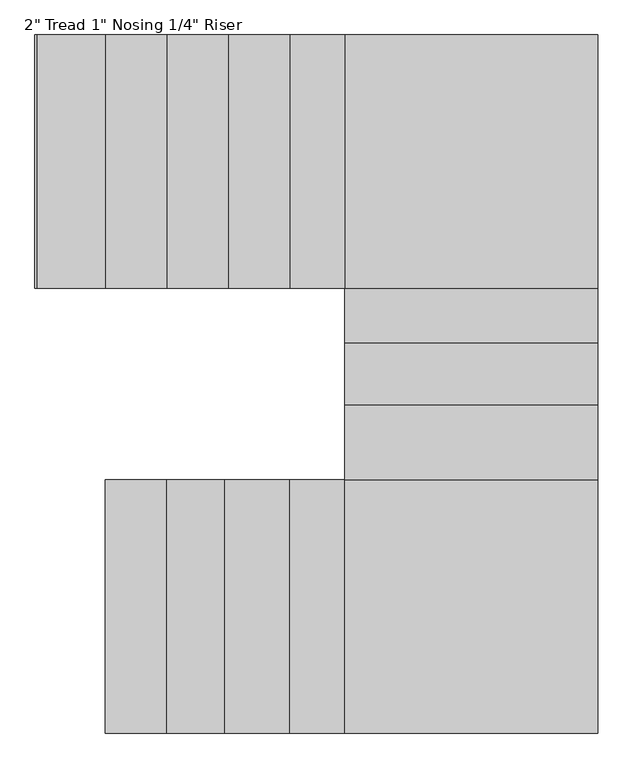
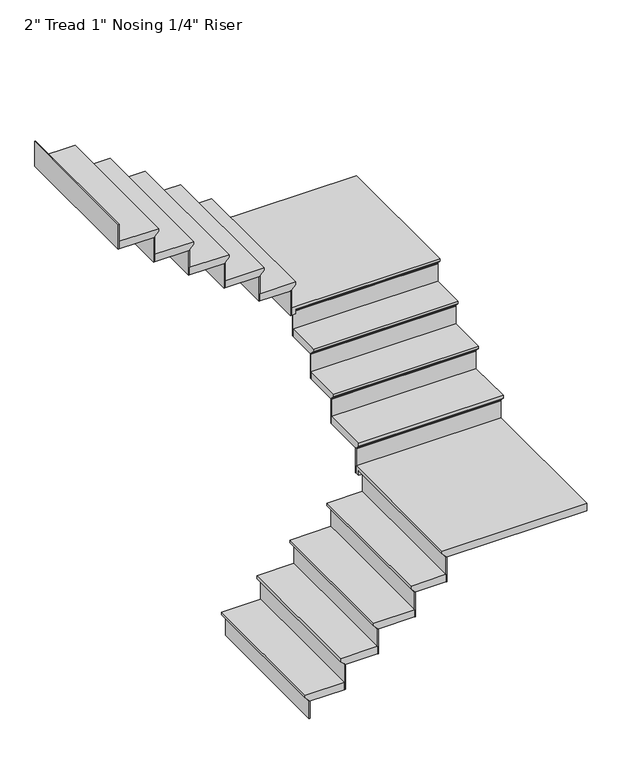
"""IFC4 building model written with IfcOpenShell, lengths in millimetres: stair flight geometry."""

from ifc_helpers import new_model, si_unit, origin, place, context, project, spatial, faceted_brep, source, transform, mapped, element, save


def stair_flight_84673ee4(model_context):
    return source(origin(), model_context, "Body", "Brep", [
        faceted_brep([(344.764115, -6141.1350571, 3350.6833333), (344.764115, -6141.1350571, 3369.7333333), (344.764115, -5201.3350571, 3369.7333333), (344.764115, -5201.3350571, 3350.6833333), (370.164115, -6141.1350571, 3325.2833333), (370.164115, -5201.3350571, 3325.2833333), (598.764115, -6141.1350571, 3369.7333333), (598.764115, -5201.3350571, 3369.7333333), (370.164115, -5201.3350571, 3318.9333333), (598.764115, -5201.3350571, 3318.9333333), (598.764115, -6141.1350571, 3318.9333333), (370.164115, -6141.1350571, 3318.9333333)], [[[0, 1, 2, 3]], [[4, 0, 3, 5]], [[2, 1, 6, 7]], [[8, 9, 10, 11]], [[2, 7, 9, 8, 5, 3]], [[8, 11, 4, 5]], [[6, 1, 0, 4, 11, 10]], [[7, 6, 10, 9]]]),
        faceted_brep([(370.164115, -6141.1350571, 3318.9333333), (370.164115, -6141.1350571, 3200.4), (376.514115, -6141.1350571, 3200.4), (376.514115, -6141.1350571, 3318.9333333), (370.164115, -5201.3350571, 3318.9333333), (376.514115, -5201.3350571, 3318.9333333), (376.514115, -5201.3350571, 3200.4), (370.164115, -5201.3350571, 3200.4)], [[[0, 1, 2, 3]], [[4, 5, 6, 7]], [[1, 0, 4, 7]], [[2, 1, 7, 6]], [[3, 2, 6, 5]], [[0, 3, 5, 4]]]),
        faceted_brep([(598.764115, -6141.1350571, 3488.2666667), (598.764115, -6141.1350571, 3318.9333333), (605.114115, -6141.1350571, 3318.9333333), (605.114115, -6141.1350571, 3488.2666667), (598.764115, -5201.3350571, 3488.2666667), (605.114115, -5201.3350571, 3488.2666667), (605.114115, -5201.3350571, 3318.9333333), (598.764115, -5201.3350571, 3318.9333333)], [[[0, 1, 2, 3]], [[4, 5, 6, 7]], [[1, 0, 4, 7]], [[2, 1, 7, 6]], [[3, 2, 6, 5]], [[0, 3, 5, 4]]]),
        faceted_brep([(573.364115, -5201.3350571, 3539.0666667), (573.364115, -6141.1350571, 3539.0666667), (814.664115, -6141.1350571, 3539.0666667), (814.664115, -5201.3350571, 3539.0666667), (598.764115, -5201.3350571, 3488.2666667), (814.664115, -5201.3350571, 3488.2666667), (814.664115, -6141.1350571, 3488.2666667), (598.764115, -6141.1350571, 3488.2666667), (598.764115, -5201.3350571, 3494.6166667), (573.364115, -5201.3350571, 3520.0166667), (598.764115, -6141.1350571, 3494.6166667), (573.364115, -6141.1350571, 3520.0166667)], [[[0, 1, 2, 3]], [[4, 5, 6, 7]], [[0, 3, 5, 4, 8, 9]], [[4, 7, 10, 8]], [[2, 1, 11, 10, 7, 6]], [[3, 2, 6, 5]], [[11, 1, 0, 9]], [[10, 11, 9, 8]]]),
        faceted_brep([(814.664115, -6141.1350571, 3657.6), (814.664115, -6141.1350571, 3488.2666667), (821.014115, -6141.1350571, 3488.2666667), (821.014115, -6141.1350571, 3657.6), (814.664115, -5201.3350571, 3657.6), (821.014115, -5201.3350571, 3657.6), (821.014115, -5201.3350571, 3488.2666667), (814.664115, -5201.3350571, 3488.2666667)], [[[0, 1, 2, 3]], [[4, 5, 6, 7]], [[1, 0, 4, 7]], [[2, 1, 7, 6]], [[3, 2, 6, 5]], [[0, 3, 5, 4]]]),
        faceted_brep([(789.264115, -5201.3350571, 3708.4), (789.264115, -6141.1350571, 3708.4), (1055.964115, -6141.1350571, 3708.4), (1055.964115, -5201.3350571, 3708.4), (814.664115, -5201.3350571, 3657.6), (1055.964115, -5201.3350571, 3657.6), (1055.964115, -6141.1350571, 3657.6), (814.664115, -6141.1350571, 3657.6), (814.664115, -5201.3350571, 3663.95), (789.264115, -5201.3350571, 3689.35), (814.664115, -6141.1350571, 3663.95), (789.264115, -6141.1350571, 3689.35)], [[[0, 1, 2, 3]], [[4, 5, 6, 7]], [[0, 3, 5, 4, 8, 9]], [[4, 7, 10, 8]], [[2, 1, 11, 10, 7, 6]], [[3, 2, 6, 5]], [[11, 1, 0, 9]], [[10, 11, 9, 8]]]),
        faceted_brep([(1055.964115, -6141.1350571, 3826.9333333), (1055.964115, -6141.1350571, 3657.6), (1062.314115, -6141.1350571, 3657.6), (1062.314115, -6141.1350571, 3826.9333333), (1055.964115, -5201.3350571, 3826.9333333), (1062.314115, -5201.3350571, 3826.9333333), (1062.314115, -5201.3350571, 3657.6), (1055.964115, -5201.3350571, 3657.6)], [[[0, 1, 2, 3]], [[4, 5, 6, 7]], [[1, 0, 4, 7]], [[2, 1, 7, 6]], [[3, 2, 6, 5]], [[0, 3, 5, 4]]]),
        faceted_brep([(1030.564115, -5201.3350571, 3877.7333333), (1030.564115, -6141.1350571, 3877.7333333), (1259.164115, -6141.1350571, 3877.7333333), (1259.164115, -5201.3350571, 3877.7333333), (1055.964115, -5201.3350571, 3826.9333333), (1259.164115, -5201.3350571, 3826.9333333), (1259.164115, -6141.1350571, 3826.9333333), (1055.964115, -6141.1350571, 3826.9333333), (1055.964115, -5201.3350571, 3833.2833333), (1030.564115, -5201.3350571, 3858.6833333), (1055.964115, -6141.1350571, 3833.2833333), (1030.564115, -6141.1350571, 3858.6833333)], [[[0, 1, 2, 3]], [[4, 5, 6, 7]], [[0, 3, 5, 4, 8, 9]], [[4, 7, 10, 8]], [[2, 1, 11, 10, 7, 6]], [[3, 2, 6, 5]], [[11, 1, 0, 9]], [[10, 11, 9, 8]]]),
        faceted_brep([(1259.164115, -6141.1350571, 3996.2666667), (1259.164115, -6141.1350571, 3826.9333333), (1265.514115, -6141.1350571, 3826.9333333), (1265.514115, -6141.1350571, 3996.2666667), (1259.164115, -5201.3350571, 3996.2666667), (1265.514115, -5201.3350571, 3996.2666667), (1265.514115, -5201.3350571, 3826.9333333), (1259.164115, -5201.3350571, 3826.9333333)], [[[0, 1, 2, 3]], [[4, 5, 6, 7]], [[1, 0, 4, 7]], [[2, 1, 7, 6]], [[3, 2, 6, 5]], [[0, 3, 5, 4]]]),
        faceted_brep([(2173.564115, -6141.1350571, 4047.0666667), (2173.564115, -5175.9350571, 4047.0666667), (1233.764115, -5175.9350571, 4047.0666667), (1233.764115, -6141.1350571, 4047.0666667), (1233.764115, -5201.3350571, 3996.2666667), (1233.764115, -5175.9350571, 3996.2666667), (2173.564115, -5175.9350571, 3996.2666667), (2173.564115, -6141.1350571, 3996.2666667), (1259.164115, -6141.1350571, 3996.2666667), (1259.164115, -5201.3350571, 3996.2666667), (1233.764115, -5201.3350571, 4028.0166667), (1233.764115, -6141.1350571, 4028.0166667), (1259.164115, -5201.3350571, 4002.6166667), (1259.164115, -6141.1350571, 4002.6166667)], [[[0, 1, 2, 3]], [[4, 5, 6, 7, 8, 9]], [[3, 2, 5, 4, 10, 11]], [[4, 9, 12, 10]], [[9, 8, 13, 12]], [[0, 3, 11, 13, 8, 7]], [[1, 0, 7, 6]], [[2, 1, 6, 5]], [[13, 11, 10, 12]]]),
        faceted_brep([(2173.564115, -5175.9350571, 4165.6), (2173.564115, -5175.9350571, 3996.2666667), (2173.564115, -5169.5850571, 3996.2666667), (2173.564115, -5169.5850571, 4165.6), (1233.764115, -5175.9350571, 4165.6), (1233.764115, -5169.5850571, 4165.6), (1233.764115, -5169.5850571, 3996.2666667), (1233.764115, -5175.9350571, 3996.2666667)], [[[0, 1, 2, 3]], [[4, 5, 6, 7]], [[1, 0, 4, 7]], [[2, 1, 7, 6]], [[3, 2, 6, 5]], [[0, 3, 5, 4]]]),
        faceted_brep([(1233.764115, -5201.3350571, 4216.4), (2173.564115, -5201.3350571, 4216.4), (2173.564115, -4896.5350571, 4216.4), (1233.764115, -4896.5350571, 4216.4), (1233.764115, -5175.9350571, 4165.6), (1233.764115, -4896.5350571, 4165.6), (2173.564115, -4896.5350571, 4165.6), (2173.564115, -5175.9350571, 4165.6), (1233.764115, -5175.9350571, 4171.95), (1233.764115, -5201.3350571, 4197.35), (2173.564115, -5175.9350571, 4171.95), (2173.564115, -5201.3350571, 4197.35)], [[[0, 1, 2, 3]], [[4, 5, 6, 7]], [[0, 3, 5, 4, 8, 9]], [[4, 7, 10, 8]], [[2, 1, 11, 10, 7, 6]], [[3, 2, 6, 5]], [[11, 1, 0, 9]], [[10, 11, 9, 8]]]),
        faceted_brep([(2173.564115, -4896.5350571, 4334.9333333), (2173.564115, -4896.5350571, 4165.6), (2173.564115, -4890.1850571, 4165.6), (2173.564115, -4890.1850571, 4334.9333333), (1233.764115, -4896.5350571, 4334.9333333), (1233.764115, -4890.1850571, 4334.9333333), (1233.764115, -4890.1850571, 4165.6), (1233.764115, -4896.5350571, 4165.6)], [[[0, 1, 2, 3]], [[4, 5, 6, 7]], [[1, 0, 4, 7]], [[2, 1, 7, 6]], [[3, 2, 6, 5]], [[0, 3, 5, 4]]]),
        faceted_brep([(1233.764115, -4921.9350571, 4385.7333333), (2173.564115, -4921.9350571, 4385.7333333), (2173.564115, -4667.9350571, 4385.7333333), (1233.764115, -4667.9350571, 4385.7333333), (1233.764115, -4896.5350571, 4334.9333333), (1233.764115, -4667.9350571, 4334.9333333), (2173.564115, -4667.9350571, 4334.9333333), (2173.564115, -4896.5350571, 4334.9333333), (1233.764115, -4896.5350571, 4341.2833333), (1233.764115, -4921.9350571, 4366.6833333), (2173.564115, -4896.5350571, 4341.2833333), (2173.564115, -4921.9350571, 4366.6833333)], [[[0, 1, 2, 3]], [[4, 5, 6, 7]], [[0, 3, 5, 4, 8, 9]], [[4, 7, 10, 8]], [[2, 1, 11, 10, 7, 6]], [[3, 2, 6, 5]], [[11, 1, 0, 9]], [[10, 11, 9, 8]]]),
        faceted_brep([(2173.564115, -4667.9350571, 4504.2666667), (2173.564115, -4667.9350571, 4334.9333333), (2173.564115, -4661.5850571, 4334.9333333), (2173.564115, -4661.5850571, 4504.2666667), (1233.764115, -4667.9350571, 4504.2666667), (1233.764115, -4661.5850571, 4504.2666667), (1233.764115, -4661.5850571, 4334.9333333), (1233.764115, -4667.9350571, 4334.9333333)], [[[0, 1, 2, 3]], [[4, 5, 6, 7]], [[1, 0, 4, 7]], [[2, 1, 7, 6]], [[3, 2, 6, 5]], [[0, 3, 5, 4]]]),
        faceted_brep([(1233.764115, -4693.3350571, 4555.0666667), (2173.564115, -4693.3350571, 4555.0666667), (2173.564115, -4464.7350571, 4555.0666667), (1233.764115, -4464.7350571, 4555.0666667), (1233.764115, -4667.9350571, 4504.2666667), (1233.764115, -4464.7350571, 4504.2666667), (2173.564115, -4464.7350571, 4504.2666667), (2173.564115, -4667.9350571, 4504.2666667), (1233.764115, -4667.9350571, 4510.6166667), (1233.764115, -4693.3350571, 4536.0166667), (2173.564115, -4667.9350571, 4510.6166667), (2173.564115, -4693.3350571, 4536.0166667)], [[[0, 1, 2, 3]], [[4, 5, 6, 7]], [[0, 3, 5, 4, 8, 9]], [[4, 7, 10, 8]], [[2, 1, 11, 10, 7, 6]], [[3, 2, 6, 5]], [[11, 1, 0, 9]], [[10, 11, 9, 8]]]),
        faceted_brep([(2173.564115, -4464.7350571, 4673.6), (2173.564115, -4464.7350571, 4504.2666667), (2173.564115, -4458.3850571, 4504.2666667), (2173.564115, -4458.3850571, 4673.6), (1233.764115, -4464.7350571, 4673.6), (1233.764115, -4458.3850571, 4673.6), (1233.764115, -4458.3850571, 4504.2666667), (1233.764115, -4464.7350571, 4504.2666667)], [[[0, 1, 2, 3]], [[4, 5, 6, 7]], [[1, 0, 4, 7]], [[2, 1, 7, 6]], [[3, 2, 6, 5]], [[0, 3, 5, 4]]]),
        faceted_brep([(2173.564115, -3550.3350571, 4724.4), (1208.364115, -3550.3350571, 4724.4), (1208.364115, -4490.1350571, 4724.4), (2173.564115, -4490.1350571, 4724.4), (1233.764115, -4490.1350571, 4673.6), (1208.364115, -4490.1350571, 4673.6), (1208.364115, -3550.3350571, 4673.6), (2173.564115, -3550.3350571, 4673.6), (2173.564115, -4464.7350571, 4673.6), (1233.764115, -4464.7350571, 4673.6), (1233.764115, -4490.1350571, 4705.35), (2173.564115, -4490.1350571, 4705.35), (1233.764115, -4464.7350571, 4679.95), (2173.564115, -4464.7350571, 4679.95)], [[[0, 1, 2, 3]], [[4, 5, 6, 7, 8, 9]], [[3, 2, 5, 4, 10, 11]], [[4, 9, 12, 10]], [[9, 8, 13, 12]], [[0, 3, 11, 13, 8, 7]], [[1, 0, 7, 6]], [[2, 1, 6, 5]], [[13, 11, 10, 12]]]),
        faceted_brep([(1208.364115, -3550.3350571, 4842.9333333), (1208.364115, -3550.3350571, 4673.6), (1202.014115, -3550.3350571, 4673.6), (1202.014115, -3550.3350571, 4842.9333333), (1208.364115, -4490.1350571, 4842.9333333), (1202.014115, -4490.1350571, 4842.9333333), (1202.014115, -4490.1350571, 4673.6), (1208.364115, -4490.1350571, 4673.6)], [[[0, 1, 2, 3]], [[4, 5, 6, 7]], [[1, 0, 4, 7]], [[2, 1, 7, 6]], [[3, 2, 6, 5]], [[0, 3, 5, 4]]]),
        faceted_brep([(1233.764115, -4490.1350571, 4893.7333333), (1233.764115, -3550.3350571, 4893.7333333), (1005.164115, -3550.3350571, 4893.7333333), (1005.164115, -4490.1350571, 4893.7333333), (1208.364115, -4490.1350571, 4842.9333333), (1005.164115, -4490.1350571, 4842.9333333), (1005.164115, -3550.3350571, 4842.9333333), (1208.364115, -3550.3350571, 4842.9333333), (1208.364115, -4490.1350571, 4849.2833333), (1233.764115, -4490.1350571, 4874.6833333), (1208.364115, -3550.3350571, 4849.2833333), (1233.764115, -3550.3350571, 4874.6833333)], [[[0, 1, 2, 3]], [[4, 5, 6, 7]], [[0, 3, 5, 4, 8, 9]], [[4, 7, 10, 8]], [[2, 1, 11, 10, 7, 6]], [[3, 2, 6, 5]], [[11, 1, 0, 9]], [[10, 11, 9, 8]]]),
        faceted_brep([(1005.164115, -3550.3350571, 5012.2666667), (1005.164115, -3550.3350571, 4842.9333333), (998.814115, -3550.3350571, 4842.9333333), (998.814115, -3550.3350571, 5012.2666667), (1005.164115, -4490.1350571, 5012.2666667), (998.814115, -4490.1350571, 5012.2666667), (998.814115, -4490.1350571, 4842.9333333), (1005.164115, -4490.1350571, 4842.9333333)], [[[0, 1, 2, 3]], [[4, 5, 6, 7]], [[1, 0, 4, 7]], [[2, 1, 7, 6]], [[3, 2, 6, 5]], [[0, 3, 5, 4]]]),
        faceted_brep([(1030.564115, -4490.1350571, 5063.0666667), (1030.564115, -3550.3350571, 5063.0666667), (776.564115, -3550.3350571, 5063.0666667), (776.564115, -4490.1350571, 5063.0666667), (1005.164115, -4490.1350571, 5012.2666667), (776.564115, -4490.1350571, 5012.2666667), (776.564115, -3550.3350571, 5012.2666667), (1005.164115, -3550.3350571, 5012.2666667), (1005.164115, -4490.1350571, 5018.6166667), (1030.564115, -4490.1350571, 5044.0166667), (1005.164115, -3550.3350571, 5018.6166667), (1030.564115, -3550.3350571, 5044.0166667)], [[[0, 1, 2, 3]], [[4, 5, 6, 7]], [[0, 3, 5, 4, 8, 9]], [[4, 7, 10, 8]], [[2, 1, 11, 10, 7, 6]], [[3, 2, 6, 5]], [[11, 1, 0, 9]], [[10, 11, 9, 8]]]),
        faceted_brep([(776.564115, -3550.3350571, 5181.6), (776.564115, -3550.3350571, 5012.2666667), (770.214115, -3550.3350571, 5012.2666667), (770.214115, -3550.3350571, 5181.6), (776.564115, -4490.1350571, 5181.6), (770.214115, -4490.1350571, 5181.6), (770.214115, -4490.1350571, 5012.2666667), (776.564115, -4490.1350571, 5012.2666667)], [[[0, 1, 2, 3]], [[4, 5, 6, 7]], [[1, 0, 4, 7]], [[2, 1, 7, 6]], [[3, 2, 6, 5]], [[0, 3, 5, 4]]]),
        faceted_brep([(801.964115, -4490.1350571, 5232.4), (801.964115, -3550.3350571, 5232.4), (547.964115, -3550.3350571, 5232.4), (547.964115, -4490.1350571, 5232.4), (776.564115, -4490.1350571, 5181.6), (547.964115, -4490.1350571, 5181.6), (547.964115, -3550.3350571, 5181.6), (776.564115, -3550.3350571, 5181.6), (776.564115, -4490.1350571, 5187.95), (801.964115, -4490.1350571, 5213.35), (776.564115, -3550.3350571, 5187.95), (801.964115, -3550.3350571, 5213.35)], [[[0, 1, 2, 3]], [[4, 5, 6, 7]], [[0, 3, 5, 4, 8, 9]], [[4, 7, 10, 8]], [[2, 1, 11, 10, 7, 6]], [[3, 2, 6, 5]], [[11, 1, 0, 9]], [[10, 11, 9, 8]]]),
        faceted_brep([(547.964115, -3550.3350571, 5350.9333333), (547.964115, -3550.3350571, 5181.6), (541.614115, -3550.3350571, 5181.6), (541.614115, -3550.3350571, 5350.9333333), (547.964115, -4490.1350571, 5350.9333333), (541.614115, -4490.1350571, 5350.9333333), (541.614115, -4490.1350571, 5181.6), (547.964115, -4490.1350571, 5181.6)], [[[0, 1, 2, 3]], [[4, 5, 6, 7]], [[1, 0, 4, 7]], [[2, 1, 7, 6]], [[3, 2, 6, 5]], [[0, 3, 5, 4]]]),
        faceted_brep([(573.364115, -4490.1350571, 5401.7333333), (573.364115, -3550.3350571, 5401.7333333), (319.364115, -3550.3350571, 5401.7333333), (319.364115, -4490.1350571, 5401.7333333), (547.964115, -4490.1350571, 5350.9333333), (319.364115, -4490.1350571, 5350.9333333), (319.364115, -3550.3350571, 5350.9333333), (547.964115, -3550.3350571, 5350.9333333), (547.964115, -4490.1350571, 5357.2833333), (573.364115, -4490.1350571, 5382.6833333), (547.964115, -3550.3350571, 5357.2833333), (573.364115, -3550.3350571, 5382.6833333)], [[[0, 1, 2, 3]], [[4, 5, 6, 7]], [[0, 3, 5, 4, 8, 9]], [[4, 7, 10, 8]], [[2, 1, 11, 10, 7, 6]], [[3, 2, 6, 5]], [[11, 1, 0, 9]], [[10, 11, 9, 8]]]),
        faceted_brep([(319.364115, -3550.3350571, 5520.2666667), (319.364115, -3550.3350571, 5350.9333333), (313.014115, -3550.3350571, 5350.9333333), (313.014115, -3550.3350571, 5520.2666667), (319.364115, -4490.1350571, 5520.2666667), (313.014115, -4490.1350571, 5520.2666667), (313.014115, -4490.1350571, 5350.9333333), (319.364115, -4490.1350571, 5350.9333333)], [[[0, 1, 2, 3]], [[4, 5, 6, 7]], [[1, 0, 4, 7]], [[2, 1, 7, 6]], [[3, 2, 6, 5]], [[0, 3, 5, 4]]]),
        faceted_brep([(90.764115, -3550.3350571, 5689.6), (90.764115, -3550.3350571, 5520.2666667), (84.414115, -3550.3350571, 5520.2666667), (84.414115, -3550.3350571, 5689.6), (90.764115, -4490.1350571, 5689.6), (84.414115, -4490.1350571, 5689.6), (84.414115, -4490.1350571, 5520.2666667), (90.764115, -4490.1350571, 5520.2666667)], [[[0, 1, 2, 3]], [[4, 5, 6, 7]], [[1, 0, 4, 7]], [[2, 1, 7, 6]], [[3, 2, 6, 5]], [[0, 3, 5, 4]]]),
        faceted_brep([(344.764115, -4490.1350571, 5571.0666667), (344.764115, -3550.3350571, 5571.0666667), (90.764115, -3550.3350571, 5571.0666667), (90.764115, -4490.1350571, 5571.0666667), (319.364115, -4490.1350571, 5520.2666667), (90.764115, -4490.1350571, 5520.2666667), (90.764115, -3550.3350571, 5520.2666667), (319.364115, -3550.3350571, 5520.2666667), (319.364115, -4490.1350571, 5526.6166667), (344.764115, -4490.1350571, 5552.0166667), (319.364115, -3550.3350571, 5526.6166667), (344.764115, -3550.3350571, 5552.0166667)], [[[0, 1, 2, 3]], [[4, 5, 6, 7]], [[0, 3, 5, 4, 8, 9]], [[4, 7, 10, 8]], [[2, 1, 11, 10, 7, 6]], [[3, 2, 6, 5]], [[11, 1, 0, 9]], [[10, 11, 9, 8]]]),
    ])


if __name__ == "__main__":
    model = new_model("IFC4")
    model_context = context("Model", 3, world=origin())
    ifc_project = project(units=[si_unit("LENGTHUNIT", "METRE", prefix="MILLI")], contexts=[model_context])
    site = spatial("IfcSite", under=ifc_project)
    building = spatial("IfcBuilding", under=site)
    placement = place(None, origin())
    stair_flight_shape = stair_flight_84673ee4(model_context)
    element("IfcStairFlight", 1, ObjectType="2\" Tread 1\" Nosing 1/4\" Riser", at=placement, inside=building, context=model_context, shape_type="MappedRepresentation", body=[
        mapped(stair_flight_shape, transform((0.0, 0.0, 0.0), x_axis=(1.0, 0.0, 0.0), y_axis=(0.0, 1.0, 0.0), z_axis=(0.0, 0.0, 1.0))),
    ])
    save(model, "model.ifc")
